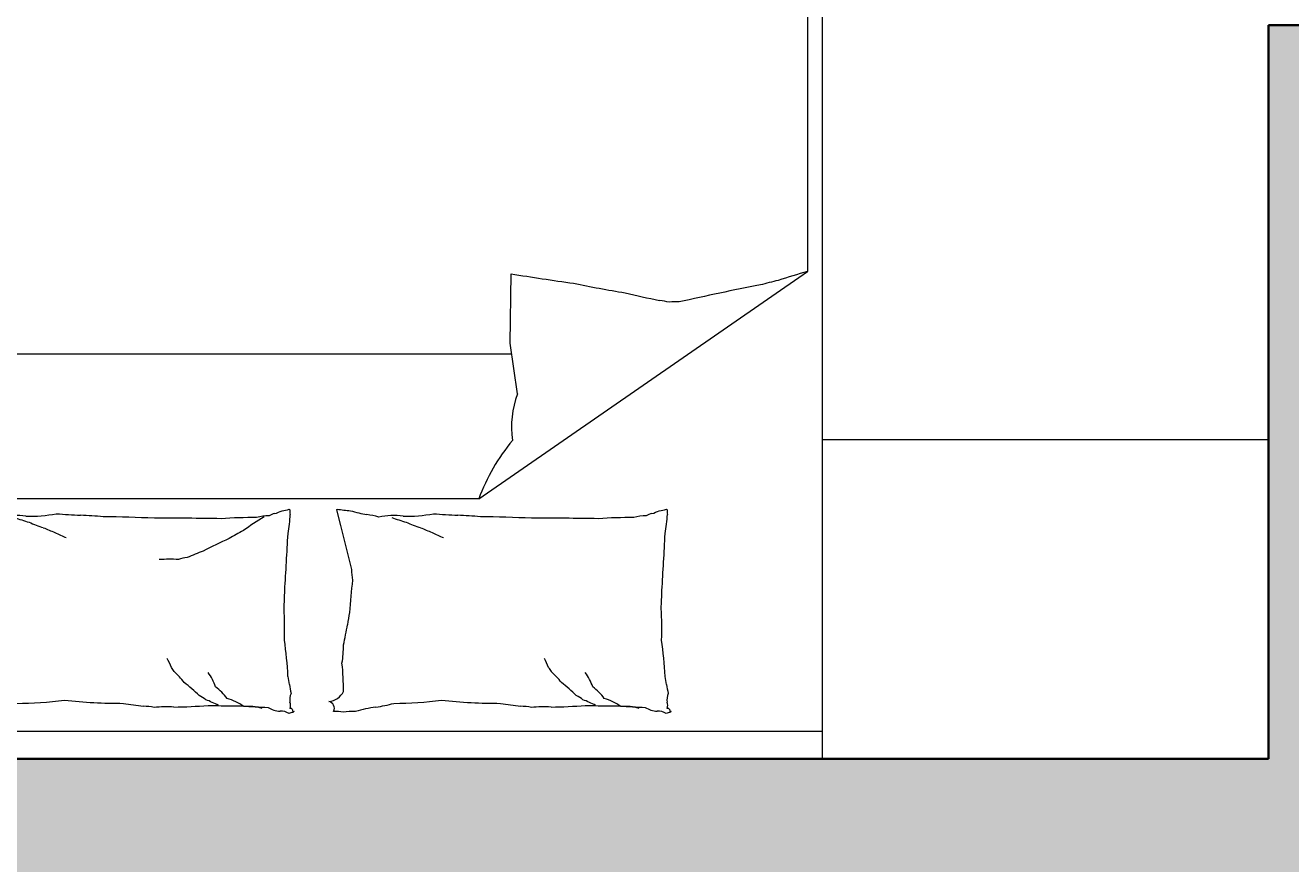
# Model space of a CAD drawing. Units: inches. Extents: x 84 to 1044, y -280 to 906.
# Tile 97 of 105: x 733 to 826, y 512 to 574. Entities that reach past the tile are written whole.
import ezdxf

# ---------------------------------------------------------------- set-up
doc = ezdxf.new("R2010")
doc.units = ezdxf.units.IN
for name, color, linetype, lineweight in [('A-ANNO-DIMS', 2, 'Continuous', 18), ('A-FURN', 8, 'Continuous', 15), ('WALL', 250, 'Continuous', 35)]:
    doc.layers.add(name, color=color, linetype=linetype, lineweight=lineweight)
doc.layers.add('A-WALL-PATT', color=251, linetype='Continuous', lineweight=9, true_color=0x636466)
doc.styles.get("Standard").update_dxf_attribs({"font": 'arial.ttf'})
doc.dimstyles.get("Standard").update_dxf_attribs({"dimtxt": 0.18, "dimasz": 0.18, "dimexe": 0.18, "dimexo": 0.0625, "dimgap": 0.09, "dimtad": 0, "dimtih": 1, "dimtoh": 1, "dimdec": 4, "dimzin": 0, "dimdsep": 46, "dimtxsty": 'Standard', "dimcen": 0.09, "dimadec": 0, "dimazin": 0, "dimtfac": 1, "dimtdec": 4, "dimtofl": 0, "dimtmove": 0, "dimatfit": 3, "dimfxl": 1, "dimtolj": 1, "dimtzin": 0, "dimarcsym": 0})

# ---------------------------------------------------------------- blocks, each defined once
blk = doc.blocks.new('BED-DOUBLE-NIGHTSTANDS')
for p, q in [((110.06, 77.08), (110.06, 35.877)), ((85.85, 19.136), (110.06, 35.877)), ((88.156, 30.614), (88.225, 35.712)), ((88.691, 26.877), (88.156, 30.614)), ((34.629, 29.814), (88.271, 29.814)), ((85.85, 19.136), (34.629, 19.136)), ((75.377, 18.345), (75.671, 17.169)), ((75.671, 17.169), (76.48, 13.934)), ((32.834, 2.051), (111.174, 2.051))]:
    blk.add_line(p, q)
for points in [[(32.834, 78.34), (32.834, 0), (111.174, 0), (111.174, 78.34)], [(144.004, 23.502), (144.004, 0), (111.174, 0), (111.174, 23.502)]]:
    blk.add_lwpolyline(points, close=True)
for centre, radius, start, end in [((112.65, 181.749), 148.065, 260.50498, 262.308), ((129.796, -33.244), 71.883, 105.93519, 107.73639), ((113.343, 134.289), 101.371, 258.32586, 260.50498), ((136.223, -121.541), 159.209, 100.72756, 102.92554), ((113.657, 10.125), 25.75, 102.92554, 105.93519), ((119.108, 130.251), 98.543, 256.8096, 258.32586), ((98.145, 26.21), 7.605, 76.8096, 82.26962), ((100.304, 31.378), 2.277, 82.26962, 100.72756), ((95.314, 24.447), 7.055, 159.85116, 188.13558), ((99.642, 14.075), 14.691, 140.35546, 159.85116), ((51.852, 12.199), 5.715, 83.56595, 101.55856), ((61.275, 45.057), 28.934, 250.57202, 252.80178), ((52.925, 26.879), 9.011, 267.25094, 281.55856), ((59.16, 72.897), 55.025, 265.38242, 267.25094), ((54.352, -29.664), 47.649, 85.38242, 87.39037), ((55.957, -113.848), 131.697, 87.39037, 89.02962), ((63.074, -206.279), 223.994, 89.02962, 90.28654), ((69.71, -27.823), 45.594, 90.28654, 93.57397), ((85.211, -6.338), 28.54, 122.13498, 125.82629), ((70.754, 12.201), 5.714, 93.57397, 102.86904), ((71.211, 16.327), 1.774, 102.86904, 117.28412), ((69.977, 20.942), 3.005, 286.22115, 297.28412), ((70.93, 21.671), 3.427, 277.12039, 286.22115), ((59.406, 18.765), 12.581, 350.00164, 356.49514), ((71.936, 18.396), 0.0517, 196.69777, 277.12039), ((72.688, 18.213), 0.757, 170.00164, 196.69777), ((75.379, 18.38), 0.0359, 265.91706, 14.04494), ((77.162, 28.85), 10.605, 260.5159, 265.91706), ((79.095, 26.856), 8.996, 252.61359, 260.5159), ((77.087, 13.323), 4.69, 72.61359, 83.56595), ((79.633, 12.199), 5.715, 83.56595, 101.55856), ((89.056, 45.057), 28.934, 250.57202, 252.80178), ((80.706, 26.879), 9.011, 267.25094, 281.55856), ((86.941, 72.897), 55.025, 265.38242, 267.25094), ((82.133, -29.664), 47.649, 85.38242, 87.39037), ((83.738, -113.848), 131.697, 87.39037, 89.02962), ((90.855, -206.279), 223.994, 89.02962, 90.28654), ((97.49, -27.823), 45.594, 90.28654, 93.57397), ((98.535, 12.201), 5.714, 93.57397, 102.86904), ((98.992, 16.327), 1.774, 102.86904, 117.28412), ((97.757, 20.942), 3.005, 286.22115, 297.28412), ((98.71, 21.671), 3.427, 277.12039, 286.22115), ((87.187, 18.765), 12.581, 350.00164, 356.49514), ((99.717, 18.396), 0.0517, 196.69777, 277.12039), ((100.469, 18.213), 0.757, 170.00164, 196.69777), ((63.398, 44.308), 28.934, 248.34226, 250.57202), ((65.304, 43.558), 28.934, 246.51559, 248.34226), ((73.97, 5.843), 12.246, 116.49848, 122.13498), ((91.179, 44.308), 28.934, 248.34226, 250.57202), ((93.085, 43.558), 28.934, 246.51559, 248.34226), ((66.996, 42.823), 28.934, 244.68893, 246.51559), ((90.567, -34.908), 56.103, 114.32653, 116.49848), ((-461.55, 45.045), 534.105, 356.49514, 356.94504), ((94.777, 42.823), 28.934, 244.68893, 246.51559), ((-433.769, 45.045), 534.105, 356.49514, 356.94504), ((72.542, -3.267), 19.845, 110.67428, 114.32653), ((63.066, 4.04), 10.656, 86.4448, 94.08277), ((64.528, 12.551), 2.271, 94.08277, 110.67428), ((102.109, 9.574), 25.804, 171.99495, 177.33512), ((79.129, 13.811), 2.652, 177.33512, 194.04519), ((18.101, 13.917), 53.476, 356.94504, 358.36691), ((45.882, 13.917), 53.476, 356.94504, 358.36691), ((44.962, 9.505), 26.586, 358.36691, 3.36875), ((88.474, 8.149), 12.422, 167.80162, 171.99495), ((72.742, 9.505), 26.586, 358.36691, 3.36875), ((42.117, 15.691), 34.549, 347.80162, 350.31563), ((36.093, 3.968), 35.764, 3.36875, 7.6809), ((67.896, 8.39), 7.99, 350.31563, 0), ((63.874, 3.968), 35.764, 3.36875, 7.6809), ((55.992, 3.673), 7.841, 23.00277, 28.31676), ((61.71, 5.52), 1.932, 28.31676, 39.03494), ((56.621, 4.955), 19.265, 0, 6.23236), ((83.773, 3.673), 7.841, 23.00277, 28.31676), ((89.491, 5.52), 1.932, 28.31676, 39.03494), ((57.304, 0.071), 8.821, 39.03494, 46.18849), ((54.629, -6.398), 15.341, 46.18849, 51.61143), ((62.775, 4.069), 3.886, 18.43965, 36.17665), ((64.2, 4.439), 7.769, 7.6809, 12.10946), ((85.084, 0.071), 8.821, 39.03494, 46.18849), ((82.41, -6.398), 15.341, 46.18849, 51.61143), ((90.555, 4.069), 3.886, 18.43965, 36.17665), ((91.981, 4.439), 7.769, 7.6809, 12.10946), ((63.873, 1.999), 3.008, 51.61143, 62.76041), ((64.172, 2.158), 3.886, 36.17665, 53.91364), ((81.439, 6.841), 9.637, 188.13348, 192.10946), ((73.212, 4.35), 1.284, 158.57902, 188.13348), ((74.694, 5.566), 1.339, 274.40021, 333.41948), ((91.653, 1.999), 3.008, 51.61143, 62.76041), ((91.953, 2.158), 3.886, 36.17665, 53.91364), ((109.22, 6.841), 9.637, 188.13348, 192.10946), ((100.993, 4.35), 1.284, 158.57902, 188.13348), ((51.809, 30.83), 26.741, 270, 277.54685), ((59.678, 45.178), 41.089, 263.9133, 270), ((63.346, 24.494), 20.732, 259.81012, 263.9133), ((60.883, -2.084), 5.969, 79.81012, 87.46141), ((62.889, -7.517), 11.348, 87.46141, 94.80185), ((63.048, 38.021), 34.204, 270.57574, 274.80185), ((62.476, -4.21), 9.167, 62.76041, 69.13972), ((67.86, 62.436), 58.531, 268.09211, 270.57574), ((66.242, 0.715), 3.886, 53.91364, 74.06476), ((71.395, 35.923), 32.15, 264.74081, 268.09211), ((68.816, -0.02), 3.886, 74.06476, 94.21588), ((71.401, 5.607), 2.112, 239.34875, 264.74081), ((71.374, 3.94), 0.611, 338.57902, 21.9904), ((74.696, 3.726), 0.514, 333.41948, 78.72762), ((80.013, -7.993), 11.938, 98.43719, 105.74398), ((77.016, 13.221), 9.489, 277.54685, 285.74398), ((79.59, 30.83), 26.741, 270, 277.54685), ((87.459, 45.178), 41.089, 263.9133, 270), ((91.127, 24.494), 20.732, 259.81012, 263.9133), ((88.664, -2.084), 5.969, 79.81012, 87.46141), ((90.67, -7.517), 11.348, 87.46141, 94.80185), ((90.829, 38.021), 34.204, 270.57574, 274.80185), ((90.257, -4.21), 9.167, 62.76041, 69.13972), ((95.641, 62.436), 58.531, 268.09211, 270.57574), ((94.023, 0.715), 3.886, 53.91364, 74.06476), ((99.176, 35.923), 32.15, 264.74081, 268.09211), ((96.597, -0.02), 3.886, 74.06476, 94.21588), ((99.182, 5.607), 2.112, 239.34875, 264.74081), ((99.155, 3.94), 0.611, 338.57902, 21.9904), ((71.293, 2.376), 1.131, 59.34875, 94.30254), ((72.234, 2.436), 0.984, 94.30254, 111.7883), ((71.977, 3.553), 0.168, 21.9904, 101.89306), ((72.218, 3.585), 0.0908, 160.43603, 281.89306), ((72.287, 3.372), 0.134, 111.7883, 160.43603), ((75.156, -0.045), 3.541, 78.72762, 90), ((76.774, -2.815), 6.312, 90, 98.43719), ((99.073, 2.376), 1.131, 59.34875, 94.30254), ((100.015, 2.436), 0.984, 94.30254, 111.7883), ((99.758, 3.553), 0.168, 21.9904, 101.89306), ((99.999, 3.585), 0.0908, 160.43603, 281.89306), ((100.068, 3.372), 0.134, 111.7883, 160.43603)]:
    blk.add_arc(centre, radius, start, end)
blk = doc.blocks.new('*D62')
at = {"layer": 'A-ANNO-DIMS', "color": 0, "lineweight": -2, "transparency": 16777216}
for p, q in [((203.179, 709.183), (203.179, 905.9)), ((203.359, 905.72), (549.232, 905.72)), ((895.894, 905.72), (550.021, 905.72)), ((896.074, 400.183), (896.074, 905.9))]:
    blk.add_line(p, q, dxfattribs=at)
at = {"layer": 'A-ANNO-DIMS', "color": 0, "transparency": 16777216}
for points in [[(203.359, 905.75), (203.359, 905.69), (203.179, 905.72)], [(895.894, 905.75), (895.894, 905.69), (896.074, 905.72)]]:
    blk.add_solid(points, dxfattribs=at)
at = {"layer": 'Defpoints', "color": 0, "transparency": 16777216}
for p in [(896.074, 905.72), (203.179, 709.12), (896.074, 400.12)]:
    blk.add_point(p, dxfattribs=at)
at = {"layer": 'A-ANNO-DIMS', "color": 0, "transparency": 16777216, "insert": (549.627, 905.72), "char_height": 0.18, "attachment_point": 5}
blk.add_mtext('\\A1;692.9', dxfattribs=at)

msp = doc.modelspace()

# ---------------------------------------------------------------- hatches: boundary and pattern name
at = {"layer": 'A-WALL-PATT', "transparency": 33554597}
h = msp.add_hatch(color=256, dxfattribs=at)
h.dxf.hatch_style = 1
h.paths.add_polyline_path([(671.074, 100.12), (647.074, 100.12), (647.074, 160.12), (641.074, 160.12), (620.824, 160.12), (620.824, 151.12), (638.074, 151.12), (638.074, 91.12), (671.074, 91.12)])
h.paths.add_polyline_path([(791.074, 100.12), (743.074, 100.12), (743.074, 91.12), (791.074, 91.12)])
h.paths.add_polyline_path([(896.074, 346.12), (887.074, 346.12), (887.074, 334.12), (870.955, 334.12), (833.074, 334.12), (804.574, 334.12), (804.574, 328.12), (887.074, 328.12), (887.074, 100.12), (863.074, 100.12), (863.074, 91.12), (896.074, 91.12)])
h.paths.add_polyline_path([(507.574, 154.729), (507.574, 160.12), (464.074, 160.12), (464.074, 247.12), (641.074, 247.12), (641.074, 208.12), (647.074, 208.12), (647.074, 328.12), (659.074, 328.12), (659.074, 334.12), (617.074, 334.12), (617.074, 328.12), (641.074, 328.12), (641.074, 256.12), (545.074, 256.12), (545.074, 328.12), (569.074, 328.12), (569.074, 334.12), (518.074, 334.12), (518.074, 325.12), (536.074, 325.12), (536.074, 256.12), (464.074, 256.12), (464.074, 325.12), (482.074, 325.12), (482.074, 334.12), (455.074, 334.12), (455.074, 160.12), (413.127, 160.12), (413.127, 151.12), (455.074, 151.12), (455.074, 91.12), (464.074, 91.12), (464.074, 151.12), (507.574, 151.12)])
h.paths.add_polyline_path([(572.824, 160.12), (555.574, 160.12), (555.574, 151.12), (572.824, 151.12)], flags=17)
h.paths.add_polyline_path([(341.127, 160.12), (299.179, 160.12), (299.179, 211.12), (294.179, 211.12), (290.179, 211.12), (290.179, 151.12), (341.127, 151.12)])
h.paths.add_polyline_path([(299.179, 256.12), (212.179, 256.12), (212.179, 274.12), (203.179, 274.12), (203.179, 247.12), (299.179, 247.12)])
h.paths.add_polyline_path([(212.179, 514.12), (398.074, 514.12), (398.074, 519.12), (398.074, 520.12), (212.179, 520.12), (212.179, 574.12), (203.179, 574.12), (203.179, 310.12), (212.179, 310.12), (212.179, 328.12), (290.179, 328.12), (290.179, 292.12), (299.179, 292.12), (299.179, 328.12), (332.179, 328.12), (332.179, 334.12), (212.179, 334.12)])
h.paths.add_polyline_path([(287.127, 709.12), (203.179, 709.12), (203.179, 646.12), (212.179, 646.12), (212.179, 700.12), (287.127, 700.12)])
h.paths.add_polyline_path([(470.074, 709.12), (359.127, 709.12), (359.127, 700.12), (434.074, 700.12), (434.074, 574.12), (440.074, 574.12), (440.074, 622.12), (464.074, 622.12), (464.074, 628.12), (440.074, 628.12), (440.074, 700.12), (470.074, 700.12)])
h.paths.add_polyline_path([(572.074, 709.12), (506.074, 709.12), (506.074, 700.12), (536.074, 700.12), (536.074, 628.12), (494.074, 628.12), (494.074, 622.12), (536.074, 622.12), (536.074, 520.12), (440.074, 520.12), (440.074, 544.12), (434.074, 544.12), (434.074, 514.12), (644.074, 514.12), (644.074, 519.12), (644.074, 544.12), (638.074, 544.12), (638.074, 520.12), (542.074, 520.12), (542.074, 622.12), (584.074, 622.12), (584.074, 628.12), (542.074, 628.12), (542.074, 700.12), (572.074, 700.12)])
h.paths.add_polyline_path([(698.074, 709.12), (608.074, 709.12), (608.074, 700.12), (638.074, 700.12), (638.074, 628.12), (614.074, 628.12), (614.074, 622.12), (638.074, 622.12), (638.074, 574.12), (644.074, 574.12), (644.074, 700.12), (698.074, 700.12)])
h.paths.add_polyline_path([(833.074, 709.12), (770.074, 709.12), (770.074, 700.12), (824.074, 700.12), (824.074, 646.12), (833.074, 646.12)])
h.paths.add_polyline_path([(833.074, 574.12), (824.074, 574.12), (824.074, 520.12), (791.244, 520.12), (712.904, 520.12), (680.074, 520.12), (680.074, 514.12), (695.074, 514.12), (695.074, 491.62), (704.074, 491.62), (704.074, 511.12), (833.074, 511.12)])
h.paths.add_polyline_path([(704.074, 419.62), (695.074, 419.62), (695.074, 370.12), (704.074, 370.12)])
h.paths.add_polyline_path([(896.074, 400.12), (833.074, 400.12), (833.074, 364.12), (839.074, 364.12), (839.074, 394.12), (887.074, 394.12), (887.074, 382.12), (896.074, 382.12)])
h.paths.add_polyline_path([(732.574, 334.12), (695.074, 334.12), (695.074, 328.12), (732.574, 328.12)])

# ---------------------------------------------------------------- linework, layer by layer
at = {"layer": 'WALL'}
for p, q in [((824.074, 520.12), (824.074, 574.12)), ((824.074, 574.12), (833.074, 574.12)), ((824.074, 520.12), (680.074, 520.12))]:
    msp.add_line(p, q, dxfattribs=at)

# ---------------------------------------------------------------- block references
at = {"layer": 'A-FURN'}
msp.add_blockref('BED-DOUBLE-NIGHTSTANDS', (680.07, 520.12), dxfattribs=at)

# ---------------------------------------------------------------- dimensions: what is measured, and where the dimension line sits
at = {"layer": 'A-ANNO-DIMS'}
dim = msp.add_linear_dim(base=(896.074, 905.72), p1=(203.179, 709.12), p2=(896.074, 400.12), dimstyle='Standard', override={"dimdec": 1, "dimlfac": 1, "dimrnd": 0, "dimzin": 0, "dimdsep": 46, "dimlunit": 2}, dxfattribs=at)
dim.commit()
dim.dimension.update_dxf_attribs({"geometry": '*D62', "text_midpoint": (549.627, 905.72)})

doc.saveas('drawing.dxf')
